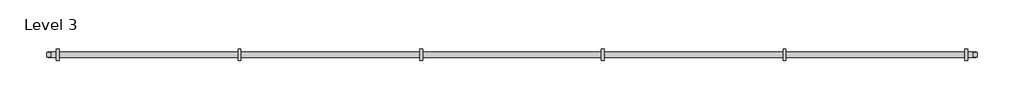
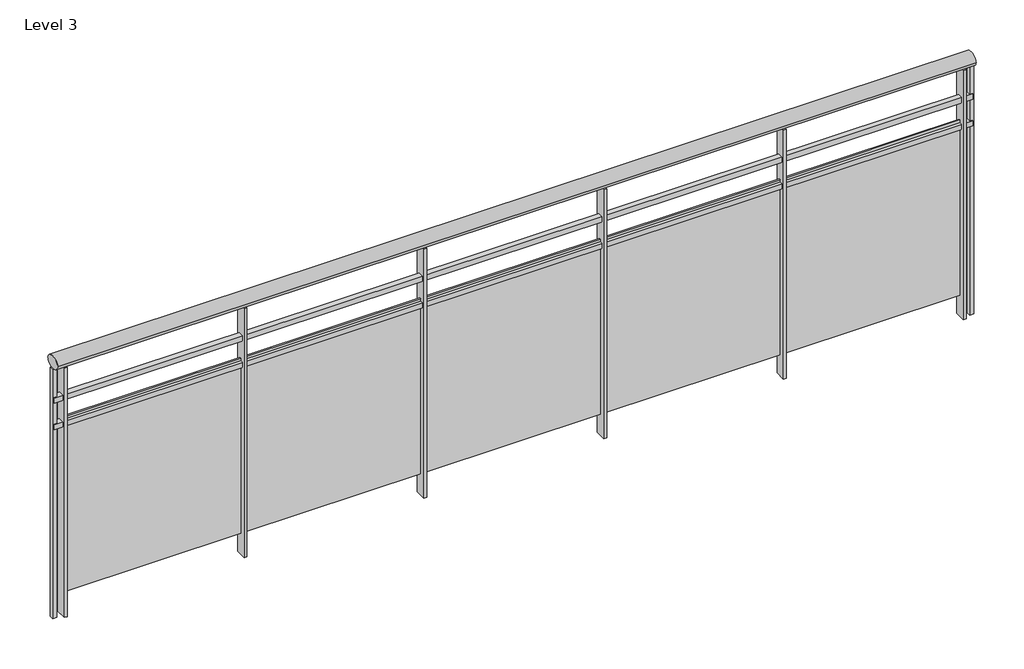
# One storey: 1 railing.
"""IFC4 building model written with IfcOpenShell, lengths in millimetres."""

from ifc_helpers import new_model, si_unit, point, frame, origin, place, context, project, spatial, polyline, ellipse_curve, trimmed, outline, extrude, element, save
from ifc_brep_helpers import plane_surface, extruded_surface, advanced_brep

model = new_model("IFC4")

# Units and contexts
model_context = context("Model", 3, world=origin())
ifc_project = project(units=[si_unit("LENGTHUNIT", "METRE", prefix="MILLI")], contexts=[model_context])

# Site, building, storey
site = spatial("IfcSite", under=ifc_project)
building = spatial("IfcBuilding", under=site)
storey = spatial("IfcBuildingStorey", under=building, Name="Level 3", Elevation=6400.8)

# Railing
placement = place(None, origin())
element("IfcRailing", 1, ObjectType="Glass Panel - Bottom Fill", at=placement, inside=storey, context=model_context, shape_type="SolidModel", body=[
    advanced_brep(
    [(-5729.1673724, -5829.5544725, 7620.0), (-5729.1673724, -5905.7544725, 7620.0), (-1576.8982041, -5829.5544725, 7620.0), (-1576.8982041, -5905.7544725, 7620.0)],
    [
        (0, 1, ellipse_curve(frame((-5729.1673724, -5867.6544725, 7620.0), z_axis=(-1.0, 0.0, 0.0), x_axis=(0.0, -1.0, 0.0)), 38.1, 28.575)),
        (1, 0, ellipse_curve(frame((-5729.1673724, -5867.6544725, 7620.0), z_axis=(-1.0, 0.0, 0.0), x_axis=(0.0, -1.0, 0.0)), 38.1, 28.575)),
        (2, 3, ellipse_curve(frame((-1576.8982041, -5867.6544725, 7620.0), z_axis=(1.0, 0.0, 0.0), x_axis=(0.0, -1.0, 0.0)), 38.1, 28.575)),
        (3, 2, ellipse_curve(frame((-1576.8982041, -5867.6544725, 7620.0), z_axis=(1.0, 0.0, 0.0), x_axis=(0.0, -1.0, 0.0)), 38.1, 28.575)),
        (0, 2),
        (3, 1),
    ],
    [
        plane_surface(frame((-5729.1673724, -5867.6544725, 7620.0), z_axis=(-1.0, 0.0, 0.0), x_axis=(0.0, 1.0, 0.0))),
        plane_surface(frame((-1576.8982041, -5867.6544725, 7620.0), z_axis=(1.0, 0.0, 0.0), x_axis=(0.0, 1.0, 0.0))),
        extruded_surface(trimmed(ellipse_curve(frame((-1576.8982041, -5867.6544725, 7620.0), z_axis=(-1.0, 0.0, 0.0), x_axis=(0.0, -1.0, 0.0)), 38.1, 28.575), [point((-1576.8982041, -5829.5544725, 7620.0))], [point((-1576.8982041, -5905.7544725, 7620.0))], True, "CARTESIAN"), (-4152.2691683, 0.0, 0.0), 4152.2691683),
        extruded_surface(trimmed(ellipse_curve(frame((-1576.8982041, -5867.6544725, 7620.0), z_axis=(-1.0, 0.0, 0.0), x_axis=(0.0, -1.0, 0.0)), 38.1, 28.575), [point((-1576.8982041, -5905.7544725, 7620.0))], [point((-1576.8982041, -5829.5544725, 7620.0))], True, "CARTESIAN"), (-4152.2691683, 0.0, 0.0), 4152.2691683),
    ],
    [
        (0, [[1, 2]]),
        (1, [[3, 4]]),
        (2, [[-1, 5, -4, 6]]),
        (3, [[-2, -6, -3, -5]]),
    ],
),
    extrude(outline(polyline([(-5729.1673724, -5880.3544725), (-5729.1673724, -5854.9544725), (-1576.8982041, -5854.9544725), (-1576.8982041, -5880.3544725), (-5729.1673724, -5880.3544725)])), frame((0.0, 0.0, 7429.5), z_axis=(0.0, 0.0, 1.0), x_axis=(1.0, 0.0, 0.0)), (0.0, 0.0, 1.0), 25.4),
    extrude(outline(polyline([(-5729.1673724, -5880.3544725), (-5729.1673724, -5854.9544725), (-1576.8982041, -5854.9544725), (-1576.8982041, -5880.3544725), (-5729.1673724, -5880.3544725)])), frame((0.0, 0.0, 7302.5), z_axis=(0.0, 0.0, 1.0), x_axis=(1.0, 0.0, 0.0)), (0.0, 0.0, 1.0), 25.4),
    extrude(outline(polyline([(-1627.3827882, -5893.0544725), (-1627.3827882, -5842.2544725), (-1614.6827882, -5842.2544725), (-1614.6827882, -5893.0544725), (-1627.3827882, -5893.0544725)])), frame((0.0, 0.0, 6400.8), z_axis=(0.0, 0.0, 1.0), x_axis=(1.0, 0.0, 0.0)), (0.0, 0.0, 1.0), 1190.625),
    extrude(outline(polyline([(-2433.8327882, -5861.1193155), (-1621.0327882, -5861.1193155), (-1621.0327882, -5867.4693155), (-2433.8327882, -5867.4693155), (-2433.8327882, -5861.1193155)])), frame((0.0, 0.0, 6502.4), z_axis=(0.0, 0.0, 1.0), x_axis=(1.0, 0.0, 0.0)), (0.0, 0.0, 1.0), 838.2),
    extrude(outline(polyline([(-2440.1827882, -5893.0544725), (-2440.1827882, -5842.2544725), (-2427.4827882, -5842.2544725), (-2427.4827882, -5893.0544725), (-2440.1827882, -5893.0544725)])), frame((0.0, 0.0, 6400.8), z_axis=(0.0, 0.0, 1.0), x_axis=(1.0, 0.0, 0.0)), (0.0, 0.0, 1.0), 1190.625),
    extrude(outline(polyline([(-3246.6327882, -5861.1193155), (-2433.8327882, -5861.1193155), (-2433.8327882, -5867.4693155), (-3246.6327882, -5867.4693155), (-3246.6327882, -5861.1193155)])), frame((0.0, 0.0, 6502.4), z_axis=(0.0, 0.0, 1.0), x_axis=(1.0, 0.0, 0.0)), (0.0, 0.0, 1.0), 838.2),
    extrude(outline(polyline([(-3252.9827882, -5893.0544725), (-3252.9827882, -5842.2544725), (-3240.2827882, -5842.2544725), (-3240.2827882, -5893.0544725), (-3252.9827882, -5893.0544725)])), frame((0.0, 0.0, 6400.8), z_axis=(0.0, 0.0, 1.0), x_axis=(1.0, 0.0, 0.0)), (0.0, 0.0, 1.0), 1190.625),
    extrude(outline(polyline([(-4059.4327882, -5861.1193155), (-3246.6327882, -5861.1193155), (-3246.6327882, -5867.4693155), (-4059.4327882, -5867.4693155), (-4059.4327882, -5861.1193155)])), frame((0.0, 0.0, 6502.4), z_axis=(0.0, 0.0, 1.0), x_axis=(1.0, 0.0, 0.0)), (0.0, 0.0, 1.0), 838.2),
    extrude(outline(polyline([(-4065.7827882, -5893.0544725), (-4065.7827882, -5842.2544725), (-4053.0827882, -5842.2544725), (-4053.0827882, -5893.0544725), (-4065.7827882, -5893.0544725)])), frame((0.0, 0.0, 6400.8), z_axis=(0.0, 0.0, 1.0), x_axis=(1.0, 0.0, 0.0)), (0.0, 0.0, 1.0), 1190.625),
    extrude(outline(polyline([(-4872.2327882, -5861.1193155), (-4059.4327882, -5861.1193155), (-4059.4327882, -5867.4693155), (-4872.2327882, -5867.4693155), (-4872.2327882, -5861.1193155)])), frame((0.0, 0.0, 6502.4), z_axis=(0.0, 0.0, 1.0), x_axis=(1.0, 0.0, 0.0)), (0.0, 0.0, 1.0), 838.2),
    extrude(outline(polyline([(-4878.5827882, -5893.0544725), (-4878.5827882, -5842.2544725), (-4865.8827882, -5842.2544725), (-4865.8827882, -5893.0544725), (-4878.5827882, -5893.0544725)])), frame((0.0, 0.0, 6400.8), z_axis=(0.0, 0.0, 1.0), x_axis=(1.0, 0.0, 0.0)), (0.0, 0.0, 1.0), 1190.625),
    extrude(outline(polyline([(-5685.0327882, -5861.1193155), (-4872.2327882, -5861.1193155), (-4872.2327882, -5867.4693155), (-5685.0327882, -5867.4693155), (-5685.0327882, -5861.1193155)])), frame((0.0, 0.0, 6502.4), z_axis=(0.0, 0.0, 1.0), x_axis=(1.0, 0.0, 0.0)), (0.0, 0.0, 1.0), 838.2),
    extrude(outline(polyline([(-5691.3827882, -5893.0544725), (-5691.3827882, -5842.2544725), (-5678.6827882, -5842.2544725), (-5678.6827882, -5893.0544725), (-5691.3827882, -5893.0544725)])), frame((0.0, 0.0, 6400.8), z_axis=(0.0, 0.0, 1.0), x_axis=(1.0, 0.0, 0.0)), (0.0, 0.0, 1.0), 1190.625),
    extrude(outline(polyline([(-1589.5982041, -5877.1794725), (-1589.5982041, -5858.1294725), (-1570.5482041, -5858.1294725), (-1570.5482041, -5877.1794725), (-1589.5982041, -5877.1794725)])), frame((0.0, 0.0, 6400.8), z_axis=(0.0, 0.0, 1.0), x_axis=(1.0, 0.0, 0.0)), (0.0, 0.0, 1.0), 1190.625),
    extrude(outline(polyline([(-5735.5173724, -5877.1794725), (-5735.5173724, -5858.1294725), (-5716.4673724, -5858.1294725), (-5716.4673724, -5877.1794725), (-5735.5173724, -5877.1794725)])), frame((0.0, 0.0, 6400.8), z_axis=(0.0, 0.0, 1.0), x_axis=(1.0, 0.0, 0.0)), (0.0, 0.0, 1.0), 1190.625),
])

save(model, "model.ifc")

# Revit data of these elements
# Type "Glass Panel - Bottom Fill"
#   Assembly Code = "C2010400"
#   built-in parameter 1008612 = 0.0416667 (stored number, unit not read)
#   built-in parameter 1008611 = 0.0416667 (stored number, unit not read)
#   built-in parameter 1008609 = 0.333333 (stored number, unit not read)
#   built-in parameter 1008604 = 0.166667 (stored number, unit not read)
#   built-in parameter 1008603 = 0.166667 (stored number, unit not read)
#   Railing Height = 4' - 0"
#   built-in parameter 1008630 = 2
#   built-in parameter 1008610 = 2
#   built-in parameter 1008618 = Baluster - Square : 3/4"
# Element 1 (IfcRailing, "Glass Panel - Bottom Fill")
#   Phase Created = New Construction
#   Materials on its faces: "Glass"
# Materials
#   "Glass": class "Glass", colour RGB 0 128 192, transparency 0.75, Description = "Soda Lime Glass", Cost = 0
